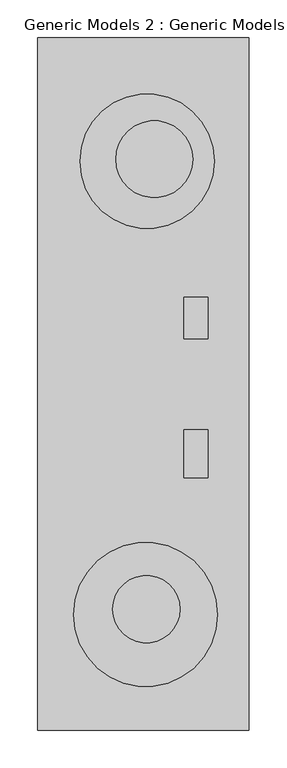
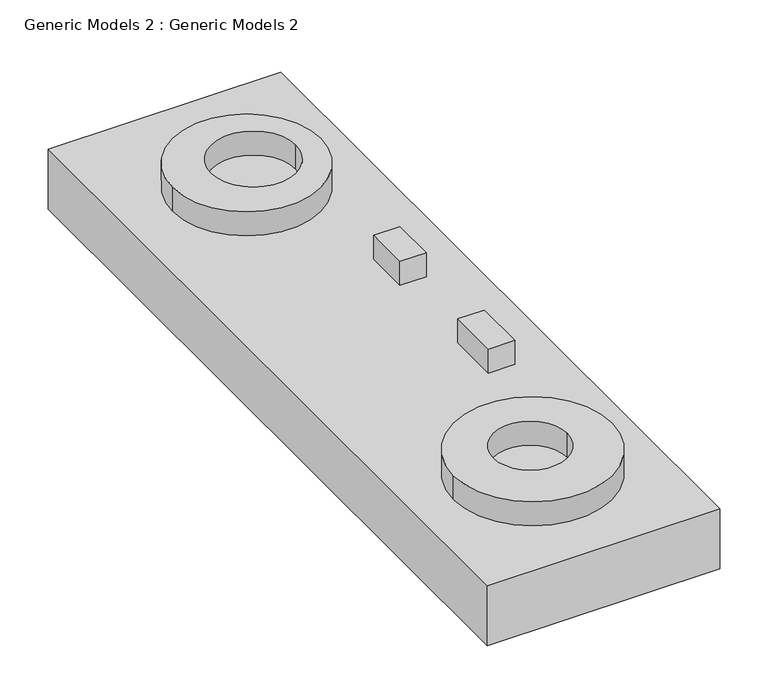
"""IFC4 building model written with IfcOpenShell, lengths in millimetres: proxy geometry, Generic Models 2 : Generic Models 2."""

from ifc_helpers import new_model, si_unit, point, frame, frame_2d, origin, place, context, project, spatial, polyline, circle_curve, trimmed, segment, composite_curve, outline, extrude, source, transform, mapped, element, save


def generic_models_2_generic_models_2_056d5301(model_context):
    return source(origin(), model_context, "Body", "SweptSolid", [
        extrude(outline(composite_curve([segment(trimmed(circle_curve(frame_2d((1523.3933799, 9558.0535459)), 88.9), [point((1434.4933799, 9558.0535459))], [point((1612.2933799, 9558.0535459))], False, "CARTESIAN"), True, "CONTINUOUS"), segment(trimmed(circle_curve(frame_2d((1523.3933799, 9558.0535459)), 88.9), [point((1612.2933799, 9558.0535459))], [point((1434.4933799, 9558.0535459))], False, "CARTESIAN"), True, "CONTINUOUS")], self_intersect=False), holes=[composite_curve([segment(trimmed(circle_curve(frame_2d((1532.9544206, 9560.6268207)), 50.8), [point((1482.1544206, 9560.6268207))], [point((1583.7544206, 9560.6268207))], True, "CARTESIAN"), True, "CONTINUOUS"), segment(trimmed(circle_curve(frame_2d((1532.9544206, 9560.6268207)), 50.8), [point((1583.7544206, 9560.6268207))], [point((1482.1544206, 9560.6268207))], True, "CARTESIAN"), True, "CONTINUOUS")], self_intersect=False)]), frame((0.0, 0.0, 1371.6), z_axis=(0.0, 0.0, 1.0), x_axis=(1.0, 0.0, 0.0)), (0.0, 0.0, 1.0), 30.48),
        extrude(outline(composite_curve([segment(trimmed(circle_curve(frame_2d((1521.4072914, 8959.2478633)), 95.25), [point((1426.1572914, 8959.2478633))], [point((1616.6572914, 8959.2478633))], False, "CARTESIAN"), True, "CONTINUOUS"), segment(trimmed(circle_curve(frame_2d((1521.4072914, 8959.2478633)), 95.25), [point((1616.6572914, 8959.2478633))], [point((1426.1572914, 8959.2478633))], False, "CARTESIAN"), True, "CONTINUOUS")], self_intersect=False), holes=[composite_curve([segment(trimmed(circle_curve(frame_2d((1522.4404639, 8966.4010131)), 44.45), [point((1477.9904639, 8966.4010131))], [point((1566.8904639, 8966.4010131))], True, "CARTESIAN"), True, "CONTINUOUS"), segment(trimmed(circle_curve(frame_2d((1522.4404639, 8966.4010131)), 44.45), [point((1566.8904639, 8966.4010131))], [point((1477.9904639, 8966.4010131))], True, "CARTESIAN"), True, "CONTINUOUS")], self_intersect=False)]), frame((0.0, 0.0, 1371.6), z_axis=(0.0, 0.0, 1.0), x_axis=(1.0, 0.0, 0.0)), (0.0, 0.0, 1.0), 30.48),
        extrude(outline(polyline([(1572.0799641, 9139.9819168), (1572.0799641, 9203.4819168), (1603.8299641, 9203.4819168), (1603.8299641, 9139.9819168), (1572.0799641, 9139.9819168)])), frame((0.0, 0.0, 1371.6), z_axis=(0.0, 0.0, 1.0), x_axis=(1.0, 0.0, 0.0)), (0.0, 0.0, 1.0), 30.48),
        extrude(outline(polyline([(1572.0799641, 9323.695103), (1572.0799641, 9378.3125367), (1603.8299641, 9378.3125367), (1603.8299641, 9323.695103), (1572.0799641, 9323.695103)])), frame((0.0, 0.0, 1371.6), z_axis=(0.0, 0.0, 1.0), x_axis=(1.0, 0.0, 0.0)), (0.0, 0.0, 1.0), 30.48),
        extrude(outline(polyline([(1378.7508072, 8806.5221058), (1378.7508072, 9720.9221058), (1658.1508072, 9720.9221058), (1658.1508072, 8806.5221058), (1378.7508072, 8806.5221058)])), frame((0.0, 0.0, 1295.4), z_axis=(0.0, 0.0, 1.0), x_axis=(1.0, 0.0, 0.0)), (0.0, 0.0, 1.0), 76.2),
    ])


if __name__ == "__main__":
    model = new_model("IFC4")
    model_context = context("Model", 3, world=origin())
    ifc_project = project(units=[si_unit("LENGTHUNIT", "METRE", prefix="MILLI")], contexts=[model_context])
    site = spatial("IfcSite", under=ifc_project)
    building = spatial("IfcBuilding", under=site)
    placement = place(None, origin())
    generic_models_2_generic_models_2_shape = generic_models_2_generic_models_2_056d5301(model_context)
    element("IfcBuildingElementProxy", 1, Name="Generic Models 2 : Generic Models 2", ObjectType="Generic Models 2 : Generic Models 2", at=placement, inside=building, context=model_context, shape_type="MappedRepresentation", body=[
        mapped(generic_models_2_generic_models_2_shape, transform((0.0, 0.0, 0.0), x_axis=(1.0, 0.0, 0.0), y_axis=(0.0, 1.0, 0.0), z_axis=(0.0, 0.0, 1.0))),
    ])
    save(model, "model.ifc")

# Revit data of these elements
# Element 1 (IfcBuildingElementProxy, "Generic Models 2 : Generic Models 2")
#   Materials on its faces: "Aluminium"
# Materials
#   "Aluminium": class "Metal", colour RGB 247 247 247, transparency 0, Description = "Aluminium 6061", Cost = 0
